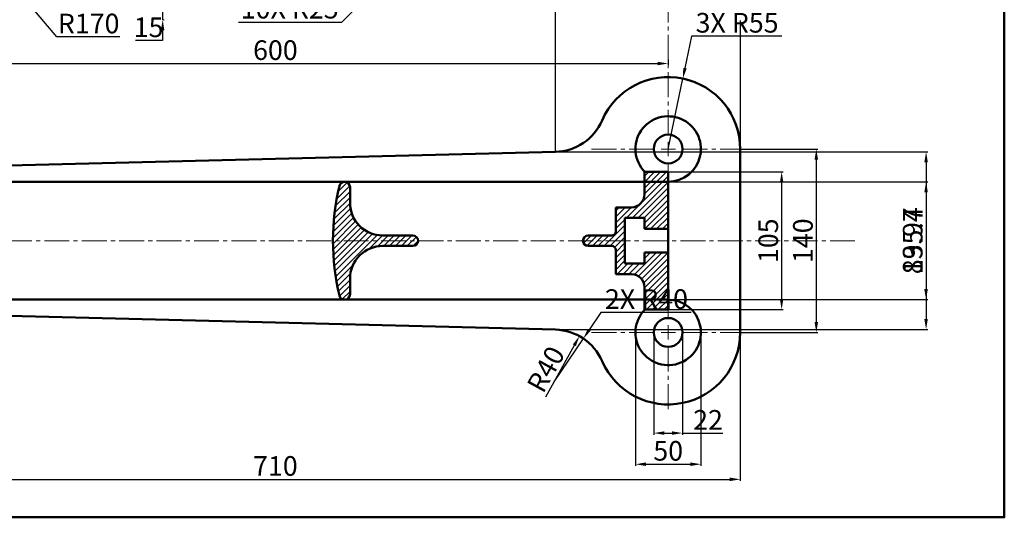
# Model space of a CAD drawing. Units: millimetres. Extents: x -60 to 1204, y -103 to 1006.
# Tile 2 of 4: x 452 to 1204, y -103 to 277. Entities that reach past the tile are written whole.
import ezdxf

# ---------------------------------------------------------------- set-up
doc = ezdxf.new("R2010")
doc.units = ezdxf.units.MM
doc.linetypes.add('CENTER2', pattern=[28.575, 19.05, -3.175, 3.175, -3.175])
for name, color, linetype, lineweight in [('M-CNTR', 1, 'CENTER2', 18), ('M-DIMS', 2, 'Continuous', 25), ('M-HATC', 8, 'Continuous', 18), ('M-OUTL', 7, 'Continuous', 50), ('M-TTLB', 7, 'Continuous', 50)]:
    doc.layers.add(name, color=color, linetype=linetype, lineweight=lineweight)
doc.styles.get("Standard").update_dxf_attribs({"font": 'arial.ttf'})
doc.dimstyles.new('ISO-25', dxfattribs={"dimtxt": 15, "dimasz": 8, "dimexe": 1.25, "dimexo": 0.625, "dimtad": 1, "dimtoh": 1, "dimdec": 0, "dimtxsty": 'Standard', "dimcen": 2.5, "dimadec": 0, "dimazin": 0, "dimtfac": 1, "dimtdec": 0, "dimtmove": 0, "dimatfit": 3, "dimfxl": 1, "dimarcsym": 0})

# ---------------------------------------------------------------- blocks, each defined once
blk = doc.blocks.new('*U2')
at = {"layer": 'M-CNTR', "color": 0, "transparency": 16777216}
for p, q in [((0, 11), (0, 257.93)), ((-58.5, 0), (-11, 0)), ((11, 0), (58.5, 0)), ((0, -58.5), (0, -11))]:
    blk.add_line(p, q, dxfattribs=at)
at = {"layer": 'M-CNTR', "color": 0, "linetype": 'Continuous', "transparency": 16777216}
for p, q in [((-5.5, 0), (5.5, 0)), ((0, -5.5), (0, 5.5))]:
    blk.add_line(p, q, dxfattribs=at)
blk = doc.blocks.new('*U3')
at = {"layer": 'M-CNTR', "color": 0, "transparency": 16777216}
for p, q in [((0, 11), (0, 58.5)), ((-58.5, 0), (-11, 0)), ((11, 0), (58.5, 0)), ((0, -58.5), (0, -11))]:
    blk.add_line(p, q, dxfattribs=at)
at = {"layer": 'M-CNTR', "color": 0, "linetype": 'Continuous', "transparency": 16777216}
for p, q in [((-5.5, 0), (5.5, 0)), ((0, -5.5), (0, 5.5))]:
    blk.add_line(p, q, dxfattribs=at)
blk = doc.blocks.new('*D33')
at = {"layer": 'Defpoints', "color": 0, "transparency": 16777216}
for p in [(561.41, 291.66), (561.41, 276.66), (561.41, 276.66)]:
    blk.add_point(p, dxfattribs=at)
at = {"layer": 'M-DIMS', "color": 0, "lineweight": -2, "transparency": 16777216}
for p, q in [((561.41, 299.66), (561.41, 307.66)), ((561.41, 291.66), (561.41, 276.66)), ((562.03, 291.66), (562.66, 291.66)), ((562.03, 276.66), (562.66, 276.66)), ((561.41, 268.66), (561.41, 260.66)), ((561.41, 260.66), (540.6, 260.66))]:
    blk.add_line(p, q, dxfattribs=at)
at = {"layer": 'M-DIMS', "color": 0, "transparency": 16777216}
for points in [[(560.08, 299.66), (562.74, 299.66), (561.41, 291.66)], [(560.08, 268.66), (562.74, 268.66), (561.41, 276.66)]]:
    blk.add_solid(points, dxfattribs=at)
at = {"layer": 'M-DIMS', "color": 0, "transparency": 16777216, "insert": (550.69, 268.95), "char_height": 15, "attachment_point": 5}
blk.add_mtext('15', dxfattribs=at)
blk = doc.blocks.new('*D51')
at = {"layer": 'Defpoints', "color": 0, "transparency": 16777216}
for p in [(347.53, 247), (947.53, 247), (947.53, 243.2)]:
    blk.add_point(p, dxfattribs=at)
at = {"layer": 'M-DIMS', "color": 0, "lineweight": -2, "transparency": 16777216}
for p, q in [((347.53, 246.37), (347.53, 241.95)), ((355.53, 243.2), (939.53, 243.2)), ((947.53, 246.37), (947.53, 241.95))]:
    blk.add_line(p, q, dxfattribs=at)
at = {"layer": 'M-DIMS', "color": 0, "transparency": 16777216}
for points in [[(355.53, 244.54), (355.53, 241.87), (347.53, 243.2)], [(939.53, 244.54), (939.53, 241.87), (947.53, 243.2)]]:
    blk.add_solid(points, dxfattribs=at)
at = {"layer": 'M-DIMS', "color": 0, "transparency": 16777216, "insert": (647.53, 251.49), "char_height": 15, "attachment_point": 5}
blk.add_mtext('600', dxfattribs=at)
blk = doc.blocks.new('*D52')
at = {"layer": 'Defpoints', "color": 0, "transparency": 16777216}
for p in [(1002.53, 177.92), (1002.53, 37.92), (1060.64, 37.92)]:
    blk.add_point(p, dxfattribs=at)
at = {"layer": 'M-DIMS', "color": 0, "lineweight": -2, "transparency": 16777216}
for p, q in [((1003.16, 177.92), (1061.89, 177.92)), ((1060.64, 169.92), (1060.64, 45.92)), ((1003.16, 37.92), (1061.89, 37.92))]:
    blk.add_line(p, q, dxfattribs=at)
at = {"layer": 'M-DIMS', "color": 0, "transparency": 16777216}
for points in [[(1059.31, 169.92), (1061.97, 169.92), (1060.64, 177.92)], [(1059.31, 45.92), (1061.97, 45.92), (1060.64, 37.92)]]:
    blk.add_solid(points, dxfattribs=at)
at = {"layer": 'M-DIMS', "color": 0, "transparency": 16777216, "insert": (1052.36, 107.92), "char_height": 15, "attachment_point": 5, "rotation": 90}
blk.add_mtext('140', dxfattribs=at)
blk = doc.blocks.new('*D53')
at = {"layer": 'Defpoints', "color": 0, "transparency": 16777216}
for p in [(947.43, 160.42), (947.43, 55.42), (1034.17, 55.42)]:
    blk.add_point(p, dxfattribs=at)
at = {"layer": 'M-DIMS', "color": 0, "lineweight": -2, "transparency": 16777216}
for p, q in [((948.05, 160.42), (1035.42, 160.42)), ((1034.17, 152.42), (1034.17, 63.42)), ((948.05, 55.42), (1035.42, 55.42))]:
    blk.add_line(p, q, dxfattribs=at)
at = {"layer": 'M-DIMS', "color": 0, "transparency": 16777216}
for points in [[(1032.84, 152.42), (1035.5, 152.42), (1034.17, 160.42)], [(1032.84, 63.42), (1035.5, 63.42), (1034.17, 55.42)]]:
    blk.add_solid(points, dxfattribs=at)
at = {"layer": 'M-DIMS', "color": 0, "transparency": 16777216, "insert": (1025.88, 107.92), "char_height": 15, "attachment_point": 5, "rotation": 90}
blk.add_mtext('105', dxfattribs=at)
blk = doc.blocks.new('*D54')
at = {"layer": 'Defpoints', "color": 0, "transparency": 16777216}
for p in [(879.7, 35.11), (860.39, 0.08)]:
    blk.add_point(p, dxfattribs=at)
at = {"layer": 'M-DIMS', "color": 0, "lineweight": -2, "transparency": 16777216}
blk.add_line((854.09, -11.34), (875.84, 28.11), dxfattribs=at)
at = {"layer": 'M-DIMS', "color": 0, "transparency": 16777216}
blk.add_solid([(874.67, 28.75), (877.01, 27.46), (879.7, 35.11)], dxfattribs=at)
at = {"layer": 'M-DIMS', "color": 0, "transparency": 16777216, "insert": (855.78, 8.88), "char_height": 15, "attachment_point": 5, "rotation": 61.13321}
blk.add_mtext('R40', dxfattribs=at)
blk = doc.blocks.new('*D55')
at = {"layer": 'Defpoints', "color": 0, "transparency": 16777216}
for p in [(936.53, 37.92), (958.53, 37.92), (958.53, -38.92)]:
    blk.add_point(p, dxfattribs=at)
at = {"layer": 'M-DIMS', "color": 0, "lineweight": -2, "transparency": 16777216}
for p, q in [((936.53, 37.3), (936.53, -40.17)), ((958.53, 37.3), (958.53, -40.17)), ((944.53, -38.92), (950.53, -38.92)), ((958.53, -38.92), (989.37, -38.92))]:
    blk.add_line(p, q, dxfattribs=at)
at = {"layer": 'M-DIMS', "color": 0, "transparency": 16777216}
for points in [[(944.53, -37.59), (944.53, -40.26), (936.53, -38.92)], [(950.53, -37.59), (950.53, -40.26), (958.53, -38.92)]]:
    blk.add_solid(points, dxfattribs=at)
at = {"layer": 'M-DIMS', "color": 0, "transparency": 16777216, "insert": (977.95, -30.77), "char_height": 15, "attachment_point": 5}
blk.add_mtext('22', dxfattribs=at)
blk = doc.blocks.new('*D56')
at = {"layer": 'Defpoints', "color": 0, "transparency": 16777216}
for p in [(922.53, 37.92), (972.53, 37.92), (972.53, -62.7)]:
    blk.add_point(p, dxfattribs=at)
at = {"layer": 'M-DIMS', "color": 0, "lineweight": -2, "transparency": 16777216}
for p, q in [((922.53, 37.3), (922.53, -63.95)), ((972.53, 37.3), (972.53, -63.95)), ((930.53, -62.7), (964.53, -62.7))]:
    blk.add_line(p, q, dxfattribs=at)
at = {"layer": 'M-DIMS', "color": 0, "transparency": 16777216}
for points in [[(930.53, -61.36), (930.53, -64.03), (922.53, -62.7)], [(964.53, -61.36), (964.53, -64.03), (972.53, -62.7)]]:
    blk.add_solid(points, dxfattribs=at)
at = {"layer": 'M-DIMS', "color": 0, "transparency": 16777216, "insert": (947.53, -54.41), "char_height": 15, "attachment_point": 5}
blk.add_mtext('50', dxfattribs=at)
blk = doc.blocks.new('RIB-SECTION')
for p, q in [((52, 74), (52, 85.91)), ((4, 49), (27, 49)), ((4, 41), (27, 41)), ((52, 16), (52, 4.09))]:
    blk.add_line(p, q)
for centre, radius, start, end in [((56.09, 85.91), 4.09, 13.44842, 180), ((-115, 45), 180, 346.55158, 13.44842), ((27, 74), 25, 270, 0), ((4, 45), 4, 90, 270), ((27, 16), 25, 0, 90), ((56.09, 4.09), 4.09, 180, 346.55158)]:
    blk.add_arc(centre, radius, start, end)
blk = doc.blocks.new('*D61')
at = {"layer": 'Defpoints', "color": 0, "transparency": 16777216}
for p in [(292.53, 276.66), (1002.53, 276.66), (1002.53, -74.23)]:
    blk.add_point(p, dxfattribs=at)
at = {"layer": 'M-DIMS', "color": 0, "lineweight": -2, "transparency": 16777216}
for p, q in [((292.53, 276.04), (292.53, -75.48)), ((1002.53, 276.04), (1002.53, -75.48)), ((300.53, -74.23), (994.53, -74.23))]:
    blk.add_line(p, q, dxfattribs=at)
at = {"layer": 'M-DIMS', "color": 0, "transparency": 16777216}
for points in [[(300.53, -72.9), (300.53, -75.56), (292.53, -74.23)], [(994.53, -72.9), (994.53, -75.56), (1002.53, -74.23)]]:
    blk.add_solid(points, dxfattribs=at)
at = {"layer": 'M-DIMS', "color": 0, "transparency": 16777216, "insert": (647.53, -65.95), "char_height": 15, "attachment_point": 5}
blk.add_mtext('710', dxfattribs=at)
blk = doc.blocks.new('*D67')
at = {"layer": 'Defpoints', "color": 0, "transparency": 16777216}
for p in [(861.39, 175.77), (861.39, 40.07), (1144.49, 40.07)]:
    blk.add_point(p, dxfattribs=at)
at = {"layer": 'M-DIMS', "color": 0, "lineweight": -2, "transparency": 16777216}
for p, q in [((862.01, 175.77), (1145.74, 175.77)), ((1144.49, 167.77), (1144.49, 48.07)), ((862.01, 40.07), (1145.74, 40.07))]:
    blk.add_line(p, q, dxfattribs=at)
at = {"layer": 'M-DIMS', "color": 0, "transparency": 16777216}
for points in [[(1143.15, 167.77), (1145.82, 167.77), (1144.49, 175.77)], [(1143.15, 48.07), (1145.82, 48.07), (1144.49, 40.07)]]:
    blk.add_solid(points, dxfattribs=at)
at = {"layer": 'M-DIMS', "color": 0, "transparency": 16777216, "insert": (1136.2, 107.92), "char_height": 15, "attachment_point": 5, "rotation": 90}
blk.add_mtext('135.7', dxfattribs=at)
blk = doc.blocks.new('*D68')
at = {"layer": 'Defpoints', "color": 0, "transparency": 16777216}
for p in [(861.39, 930.31), (861.39, 175.77), (347.53, 107.92)]:
    blk.add_point(p, dxfattribs=at)
at = {"layer": 'M-DIMS', "color": 0, "lineweight": -2, "transparency": 16777216}
for p, q in [((347.53, 108.55), (347.53, 931.56)), ((355.53, 930.31), (853.39, 930.31)), ((861.39, 176.39), (861.39, 931.56))]:
    blk.add_line(p, q, dxfattribs=at)
at = {"layer": 'M-DIMS', "color": 0, "transparency": 16777216}
for points in [[(355.53, 931.65), (355.53, 928.98), (347.53, 930.31)], [(853.39, 931.65), (853.39, 928.98), (861.39, 930.31)]]:
    blk.add_solid(points, dxfattribs=at)
at = {"layer": 'M-DIMS', "color": 0, "transparency": 16777216, "insert": (604.46, 938.6), "char_height": 15, "attachment_point": 5}
blk.add_mtext('513.9', dxfattribs=at)
blk = doc.blocks.new('*D69')
at = {"layer": 'Defpoints', "color": 0, "transparency": 16777216}
for p in [(347.53, 152.89), (347.53, 62.95), (1144.49, 62.95)]:
    blk.add_point(p, dxfattribs=at)
at = {"layer": 'M-DIMS', "color": 0, "lineweight": -2, "transparency": 16777216}
for p, q in [((348.16, 152.89), (1145.74, 152.89)), ((1144.49, 144.89), (1144.49, 70.95)), ((348.16, 62.95), (1145.74, 62.95))]:
    blk.add_line(p, q, dxfattribs=at)
at = {"layer": 'M-DIMS', "color": 0, "transparency": 16777216}
for points in [[(1143.15, 144.89), (1145.82, 144.89), (1144.49, 152.89)], [(1143.15, 70.95), (1145.82, 70.95), (1144.49, 62.95)]]:
    blk.add_solid(points, dxfattribs=at)
at = {"layer": 'M-DIMS', "color": 0, "transparency": 16777216, "insert": (1136.2, 107.92), "char_height": 15, "attachment_point": 5, "rotation": 90}
blk.add_mtext('89.94', dxfattribs=at)
blk = doc.blocks.new('*D71')
at = {"layer": 'Defpoints', "color": 0, "transparency": 16777216}
for p in [(305.45, 471.66), (414.89, 341.57)]:
    blk.add_point(p, dxfattribs=at)
at = {"layer": 'M-DIMS', "color": 0, "lineweight": -2, "transparency": 16777216}
for p, q in [((305.45, 471.66), (414.89, 341.57)), ((480.54, 263.51), (420.04, 335.45)), ((528.62, 263.51), (480.54, 263.51))]:
    blk.add_line(p, q, dxfattribs=at)
at = {"layer": 'M-DIMS', "color": 0, "transparency": 16777216}
blk.add_solid([(421.06, 336.31), (419.01, 334.59), (414.89, 341.57)], dxfattribs=at)
at = {"layer": 'M-DIMS', "color": 0, "transparency": 16777216, "insert": (504.89, 271.8), "char_height": 15, "attachment_point": 5}
blk.add_mtext('R170', dxfattribs=at)
blk = doc.blocks.new('*D73')
at = {"layer": 'Defpoints', "color": 0, "transparency": 16777216}
for p in [(958.72, 231.77), (947.53, 177.92)]:
    blk.add_point(p, dxfattribs=at)
at = {"layer": 'M-DIMS', "color": 0, "lineweight": -2, "transparency": 16777216}
for p, q in [((965.43, 264.08), (960.34, 239.6)), ((1034.23, 264.08), (965.43, 264.08)), ((947.53, 177.92), (958.72, 231.77))]:
    blk.add_line(p, q, dxfattribs=at)
at = {"layer": 'M-DIMS', "color": 0, "transparency": 16777216}
blk.add_solid([(959.04, 239.87), (961.65, 239.33), (958.72, 231.77)], dxfattribs=at)
at = {"layer": 'M-DIMS', "color": 0, "transparency": 16777216, "insert": (1000.14, 272.37), "char_height": 15, "attachment_point": 5}
blk.add_mtext('3X R55', dxfattribs=at)
blk = doc.blocks.new('*D74')
at = {"layer": 'Defpoints', "color": 0, "transparency": 16777216}
for p in [(882.75, 33.25), (860.39, 0.08)]:
    blk.add_point(p, dxfattribs=at)
at = {"layer": 'M-DIMS', "color": 0, "lineweight": -2, "transparency": 16777216}
for p, q in [((896.16, 53.15), (887.22, 39.89)), ((965.06, 53.15), (896.16, 53.15)), ((860.39, 0.08), (882.75, 33.25))]:
    blk.add_line(p, q, dxfattribs=at)
at = {"layer": 'M-DIMS', "color": 0, "transparency": 16777216}
blk.add_solid([(886.11, 40.63), (888.32, 39.14), (882.75, 33.25)], dxfattribs=at)
at = {"layer": 'M-DIMS', "color": 0, "transparency": 16777216, "insert": (930.92, 61.44), "char_height": 15, "attachment_point": 5}
blk.add_mtext('2X R40', dxfattribs=at)
blk = doc.blocks.new('*D75')
at = {"layer": 'Defpoints', "color": 0, "transparency": 16777216}
for p in [(738.13, 314.66), (720.45, 296.99)]:
    blk.add_point(p, dxfattribs=at)
at = {"layer": 'M-DIMS', "color": 0, "lineweight": -2, "transparency": 16777216}
for p, q in [((738.13, 314.66), (720.45, 296.99)), ((698.3, 274.84), (714.79, 291.33)), ((619.25, 274.84), (698.3, 274.84))]:
    blk.add_line(p, q, dxfattribs=at)
at = {"layer": 'M-DIMS', "color": 0, "transparency": 16777216}
blk.add_solid([(713.85, 292.27), (715.73, 290.39), (720.45, 296.99)], dxfattribs=at)
at = {"layer": 'M-DIMS', "color": 0, "transparency": 16777216, "insert": (658.46, 283.13), "char_height": 15, "attachment_point": 5}
blk.add_mtext('10X R25', dxfattribs=at)

msp = doc.modelspace()

# ---------------------------------------------------------------- hatches: boundary and pattern name
at = {"layer": 'M-HATC'}
h = msp.add_hatch(dxfattribs=at)
h.set_pattern_fill('ANSI31', color=256)
h.set_pattern_definition([(45, (619.5597, -678.0574), (-2.245064, 2.245064), [])])
h.paths.add_polyline_path([(919.4285, 133.4202), (907.4285, 133.4202), (907.4285, 114.9202, -0.41421356), (904.4285, 111.9202), (886.4285, 111.9202, 1), (886.4285, 103.9202), (904.4285, 103.9202, -0.41421356), (907.4285, 100.9202), (907.4285, 82.4202), (919.4285, 82.4202, -0.41421356), (929.4285, 72.4202), (929.4285, 55.4202), (947.4285, 55.4202), (947.4285, 98.9202), (929.4285, 98.9202), (929.4285, 90.4202), (914.4285, 90.4202), (914.4285, 125.4202), (929.4285, 125.4202), (929.4285, 116.9202), (947.4285, 116.9202), (947.4285, 160.4202), (929.4285, 160.4202), (929.4285, 143.4202, -0.41421356)])
h = msp.add_hatch(dxfattribs=at)
h.set_pattern_fill('ANSI31', color=256, angle=180)
h.set_pattern_definition([(225, (1494.1794, 580.49), (2.245064, -2.245064), [])])
h.paths.add_polyline_path([(691.5067, 107.9202, 0.05874724), (696.4424, 66.0576, 0.889025), (704.5067, 67.0084), (704.5067, 78.9202, -0.41421356), (729.5067, 103.9202), (752.5067, 103.9202, 0.41421356), (756.5067, 107.9202)])
h.paths.add_polyline_path([(756.5067, 107.9202, 0.41421356), (752.5067, 111.9202), (729.5067, 111.9202, -0.41421356), (704.5067, 136.9202), (704.5067, 148.8319, 0.889025), (696.4424, 149.7827, 0.05874724), (691.5067, 107.9202)])

# ---------------------------------------------------------------- linework, layer by layer
at = {"layer": 'M-CNTR'}
msp.add_line((271.0408, 107.9202), (1090.8372, 107.9202), dxfattribs=at)
at = {"layer": 'M-OUTL'}
for p, q in [((346.1577, 162.903), (861.3892, 175.7691)), ((1002.5307, 177.9202), (1002.5307, 37.9202)), ((947.4285, 160.4202), (929.4285, 160.4202)), ((929.4285, 160.4202), (929.4285, 143.4202)), ((947.4285, 160.4202), (947.4285, 116.9202)), ((700.8972, 152.892), (347.5307, 152.892)), ((700.4185, 152.9202), (947.4285, 152.9202)), ((919.4285, 133.4202), (907.4285, 133.4202)), ((907.4285, 133.4202), (907.4285, 114.9202)), ((929.4285, 125.4202), (914.4285, 125.4202)), ((914.4285, 125.4202), (914.4285, 90.4202)), ((929.4285, 116.9202), (929.4285, 125.4202)), ((929.4285, 116.9202), (947.4285, 116.9202)), ((947.4285, 116.9202), (947.4285, 98.9202)), ((886.4285, 111.9202), (904.4285, 111.9202)), ((886.4285, 103.9202), (904.4285, 103.9202)), ((907.4285, 100.9202), (907.4285, 82.4202)), ((929.4285, 98.9202), (947.4285, 98.9202)), ((929.4285, 90.4202), (929.4285, 98.9202)), ((947.4285, 98.9202), (947.4285, 55.4202)), ((914.4285, 90.4202), (929.4285, 90.4202)), ((907.4285, 82.4202), (919.4285, 82.4202)), ((929.4285, 72.4202), (929.4285, 55.4202)), ((700.8972, 62.9483), (347.5307, 62.9483)), ((699.9398, 62.9483), (947.5307, 62.9483)), ((346.1577, 52.9373), (861.3892, 40.0712)), ((947.4285, 55.4202), (929.4285, 55.4202))]:
    msp.add_line(p, q, dxfattribs=at)
for centre in [(947.5307, 177.9202), (947.5307, 37.9202)]:
    msp.add_circle(centre, 11, dxfattribs=at)
for centre, radius, start, end in [((947.5307, 177.9202), 55, 0, 156.5293976), ((860.3906, 215.7566), 40, 271.4304599, 336.5293976), ((947.5307, 177.9202), 25, 269.7656879, 224.427004), ((919.4285, 143.4202), 10, 270, 0), ((904.4285, 114.9202), 3, 270, 0), ((886.4285, 107.9202), 4, 90, 270), ((904.4285, 100.9202), 3, 0, 90), ((919.4285, 72.4202), 10, 0, 90), ((947.5307, 37.9202), 25, 135.572996, 90.2343121), ((860.3906, 0.0837), 40, 23.4706024, 88.5695401), ((947.5307, 37.9202), 55, 203.4706024, 0)]:
    msp.add_arc(centre, radius, start, end, dxfattribs=at)
at = {"layer": 'M-TTLB'}
msp.add_lwpolyline([(-59.5454, 1006.1383), (1204.2342, 1006.1383), (1204.2342, -103.2116), (-59.5454, -103.2116)], close=True, dxfattribs=at)

# ---------------------------------------------------------------- block references
at = {"layer": 'M-CNTR'}
for name, p in [('*U2', (947.5307, 177.9202)), ('*U3', (947.5307, 37.9202))]:
    msp.add_blockref(name, p, dxfattribs=at)
at = {"layer": 'M-OUTL', "rotation": 180}
msp.add_blockref('RIB-SECTION', (756.5064, 152.9191), dxfattribs=at)

# ---------------------------------------------------------------- dimensions: what is measured, and where the dimension line sits
at = {"layer": 'M-DIMS'}
for base, p1, p2, override, picture, middle in [((861.3892, 930.3142), (347.5307, 107.9202), (861.3892, 175.7691), {"dimdec": 1, "dimlfac": 1, "dimrnd": 0, "dimzin": 0, "dimdsep": 46, "dimlunit": 2}, '*D68', (604.46, 938.6029)), ((1002.5307, -74.2298), (292.5307, 276.6642), (1002.5307, 276.6642), {"dimdec": 0, "dimlfac": 1, "dimrnd": 0, "dimzin": 0, "dimdsep": 46, "dimlunit": 2}, '*D61', (647.5307, -65.9462)), ((947.5307, 243.2036), (347.5307, 246.9971), (947.5307, 246.9971), {"dimclrd": 0, "dimclre": 0, "dimclrt": 0}, '*D51', (647.5307, 251.4872)), ((972.5307, -62.6951), (922.5307, 37.9202), (972.5307, 37.9202), {"dimclrd": 0, "dimclre": 0, "dimclrt": 0}, '*D56', (947.5307, -54.4115)), ((958.5307, -38.9221), (936.5307, 37.9202), (958.5307, 37.9202), {"dimclrd": 0, "dimclre": 0, "dimclrt": 0}, '*D55', (977.9504, -30.7664))]:
    dim = msp.add_linear_dim(base=base, p1=p1, p2=p2, dimstyle='ISO-25', override=override, dxfattribs=at)
    dim.commit()
    dim.dimension.update_dxf_attribs({"geometry": picture, "text_midpoint": middle})
for center, mpoint, override, picture, middle in [((305.4532, 471.6642), (414.8855, 341.5697), {"dimdec": 0, "dimlfac": 1, "dimrnd": 0, "dimzin": 0, "dimdsep": 46, "dimlunit": 2}, '*D71', (504.8926, 263.513)), ((860.3906, 0.0837), (879.7016, 35.1135), {"dimclrd": 0, "dimclre": 0, "dimclrt": 0}, '*D54', (863.0359, 4.8822))]:
    dim = msp.add_radius_dim(center=center, mpoint=mpoint, dimstyle='ISO-25', override=override, dxfattribs=at)
    dim.commit()
    dim.dimension.update_dxf_attribs({"geometry": picture, "text_midpoint": middle, "dimtype": 164})
dim = msp.add_radius_dim(center=(738.1258, 314.6642), mpoint=(720.4478, 296.9868), text='10X <>', dimstyle='ISO-25', override={"dimdec": 0, "dimlfac": 1, "dimrnd": 0, "dimzin": 0, "dimdsep": 46, "dimlunit": 2}, dxfattribs=at)
dim.commit()
dim.dimension.update_dxf_attribs({"geometry": '*D75', "text_midpoint": (658.464, 283.1262)})
dim = msp.add_aligned_dim(p1=(561.4091, 291.6642), p2=(561.4091, 276.6642), distance=0, dimstyle='ISO-25', override={"dimclrd": 0, "dimclre": 0, "dimclrt": 0}, dxfattribs=at)
dim.commit()
dim.dimension.update_dxf_attribs({"geometry": '*D33', "text_midpoint": (550.6903, 268.9478)})
for center, mpoint, text, picture, middle in [((947.5307, 177.9202), (958.7169, 231.7706), '3X <>', '*D73', (1000.1413, 264.0809)), ((860.3906, 0.0837), (882.7469, 33.2529), '2X <>', '*D74', (930.9245, 53.1544))]:
    dim = msp.add_radius_dim(center=center, mpoint=mpoint, text=text, dimstyle='ISO-25', override={"dimdec": 0, "dimlfac": 1, "dimrnd": 0, "dimzin": 0, "dimdsep": 46, "dimlunit": 2}, dxfattribs=at)
    dim.commit()
    dim.dimension.update_dxf_attribs({"geometry": picture, "text_midpoint": middle, "dimtype": 164})
for base, p1, p2, override, picture, middle in [((1144.4872, 40.0712), (861.3892, 175.7691), (861.3892, 40.0712), {"dimdec": 1, "dimlfac": 1, "dimrnd": 0, "dimzin": 0, "dimdsep": 46, "dimlunit": 2}, '*D67', (1136.1985, 107.9202)), ((1060.6403, 37.9202), (1002.5307, 177.9202), (1002.5307, 37.9202), {"dimclrd": 0, "dimclre": 0, "dimclrt": 0}, '*D52', (1052.3567, 107.9202)), ((1034.1686, 55.4202), (947.4285, 160.4202), (947.4285, 55.4202), {"dimclrd": 0, "dimclre": 0, "dimclrt": 0}, '*D53', (1025.885, 107.9202)), ((1144.4872, 62.9483), (347.5307, 152.892), (347.5307, 62.9483), {"dimdec": 2, "dimlfac": 1, "dimrnd": 0, "dimzin": 0, "dimdsep": 46, "dimlunit": 2}, '*D69', (1136.2036, 107.9202))]:
    dim = msp.add_linear_dim(base=base, p1=p1, p2=p2, angle=90, dimstyle='ISO-25', override=override, dxfattribs=at)
    dim.commit()
    dim.dimension.update_dxf_attribs({"geometry": picture, "text_midpoint": middle})

doc.saveas('drawing.dxf')
